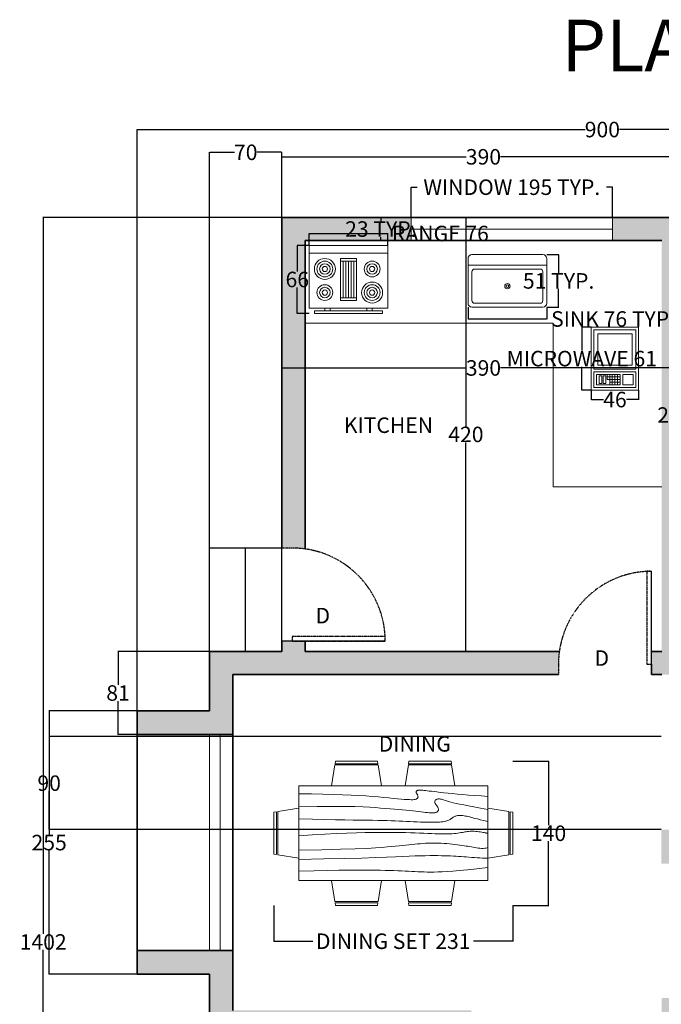
# Model space of a CAD drawing. Units: centimetres. Extents: x 355 to 1615, y 1030 to 2729.
# Tile 2 of 3: x 358 to 978, y 1776 to 2729. Entities that reach past the tile are written whole.
import ezdxf

# ---------------------------------------------------------------- set-up
doc = ezdxf.new("R2010")
doc.units = ezdxf.units.CM
doc.header["$MEASUREMENT"] = 0
doc.linetypes.add('HIDDEN', pattern=[0.375, 0.25, -0.125])
for name, color, linetype, lineweight in [('A-ANNO-DIMS', 2, 'Continuous', 18), ('A-ANNO-TEXT', 7, 'Continuous', 25), ('A-AREA-IDEN', 7, 'Continuous', 25), ('A-DOOR', 4, 'Continuous', 25), ('A-DOOR-HIDN', 4, 'HIDDEN', 25), ('A-EQPM', 8, 'Continuous', 18), ('A-FLOR-CASE', 9, 'Continuous', 20), ('A-FLOR-FIXT', 9, 'Continuous', 18), ('A-FLOR-STRS', 7, 'Continuous', 25), ('A-FURN', 8, 'Continuous', 18), ('A-GLAZ', 4, 'Continuous', 18), ('A-WALL', 7, 'Continuous', 35), ('A-WALL-PATT', 5, 'Continuous', 13)]:
    doc.layers.add(name, color=color, linetype=linetype, lineweight=lineweight)
doc.styles.get("Standard").update_dxf_attribs({"font": 'arial.ttf'})
doc.dimstyles.get("Standard").update_dxf_attribs({"dimtxt": 15, "dimasz": 0.18, "dimexe": 0.18, "dimexo": 0.0625, "dimgap": 0.09, "dimtad": 0, "dimtih": 1, "dimtoh": 1, "dimdec": 0, "dimzin": 0, "dimdsep": 46, "dimtxsty": 'Standard', "dimcen": 0.09, "dimadec": 0, "dimazin": 0, "dimtfac": 1, "dimtdec": 0, "dimtofl": 0, "dimtmove": 0, "dimatfit": 3, "dimfxl": 1, "dimtolj": 1, "dimtzin": 0, "dimarcsym": 0})

# ---------------------------------------------------------------- blocks, each defined once
blk = doc.blocks.new('*U2')
for p, q in [((0, 0), (0, -100)), ((-900, 0), (-900, -100))]:
    blk.add_line(p, q)
blk.add_lwpolyline([(0, 0), (0, 900), (-43.75, 900), (-43.75, 0)], close=True)
blk.add_arc((0, 0), 900, 90, 180)
blk = doc.blocks.new('*U3')
for p, q in [((0, 0), (0, -100)), ((-900, 0), (-900, -100))]:
    blk.add_line(p, q)
blk.add_lwpolyline([(0, 0), (0, 900), (-43.75, 900), (-43.75, 0)], close=True)
blk.add_arc((0, 0), 900, 90, 180)
blk = doc.blocks.new('Range-Oven - 30 in top')
for p, q in [((0, -3), (30, -3)), ((12, -6), (18, -6)), ((13, -20), (13, -6)), ((14, -6), (14, -20)), ((15, -20), (15, -6)), ((16, -6), (16, -20)), ((17, -20), (17, -6)), ((18, -20), (12, -20)), ((6, -24), (6, -25)), ((8, -25), (8, -24)), ((22, -25), (22, -24)), ((24, -24), (24, -25))]:
    blk.add_line(p, q)
for points in [[(0, -24), (0, 0), (30, 0), (30, -24)], [(12, -21), (12, -5), (18, -5), (18, -21)], [(2, -26), (2, -25), (28, -25), (28, -26)]]:
    blk.add_lwpolyline(points, close=True)
for centre, radius in [((6, -9), 4), ((6, -9), 3), ((6, -9), 2), ((24, -9), 3), ((24, -9), 2), ((6, -9), 1), ((24, -9), 1), ((6, -18), 3), ((24, -18), 4), ((24, -18), 3), ((6, -18), 2), ((6, -18), 1), ((24, -18), 2), ((24, -18), 1)]:
    blk.add_circle(centre, radius)
blk = doc.blocks.new('Sink-single - 30 in top')
blk.add_line((-15, -3.999996), (15, -3.999996))
for points in [[(-13.5, 0), (13.5, 0)], [(-15, -18.499996), (-15, -1.5)], [(15, -1.5), (15, -18.499996)], [(-13.5, -17.499996), (-13.5, -6.499996)], [(-12.5, -5.499996), (12.5, -5.499996)], [(13.5, -6.499996), (13.5, -17.499996)], [(12.5, -18.499996), (-12.5, -18.499996)], [(13.5, -19.999996), (-13.5, -19.999996)]]:
    blk.add_lwpolyline(points)
for radius in [1, 0.5]:
    blk.add_circle((0, -11.999996), radius)
for centre, radius, start, end in [((-13.5, -1.5), 1.5, 90, 180), ((13.5, -1.5), 1.5, 0, 90), ((-12.5, -6.499996), 1, 90, 180), ((12.5, -6.499996), 1, 0, 90), ((-13.5, -18.499996), 1.5, 180, 270), ((-12.5, -17.499996), 1, 180, 270), ((12.5, -17.499996), 1, 270, 0), ((13.5, -18.499996), 1.5, 270, 0)]:
    blk.add_arc(centre, radius, start, end)
blk = doc.blocks.new('Microwave')
for p, q in [((18, 10), (22, 10)), ((22, 9), (18, 9)), ((18, 8), (22, 8)), ((19, 7), (19, 11)), ((20, 11), (20, 7)), ((21, 7), (21, 11)), ((22, 7), (18, 7)), ((20, 6), (18, 6)), ((19, 6), (19, 7)), ((20, 7), (20, 6))]:
    blk.add_line(p, q)
for points in [[(0, 0), (0, 18), (24, 18), (24, 0)], [(1, 1), (1, 17), (16, 17), (16, 1)], [(2.5, 2.5), (2.5, 15.5), (14.5, 15.5), (14.5, 2.5)], [(17, 1), (17, 17), (23, 17), (23, 1)], [(18, 12), (18, 16), (22, 16), (22, 12)], [(18, 2), (18, 11), (22, 11), (22, 2)], [(18.5, 4.5), (18.5, 5.5), (21.5, 5.5), (21.5, 4.5)], [(18.5, 3), (18.5, 4), (21.5, 4), (21.5, 3)]]:
    blk.add_lwpolyline(points, close=True)
blk = doc.blocks.new('*D8')
at = {"layer": 'A-ANNO-DIMS', "color": 0, "lineweight": -2, "transparency": 16777216}
for p, q in [((611.23, 2537.61), (611.23, 2391.81)), ((1001.23, 2537.61), (1001.23, 2391.81)), ((611.41, 2391.99), (789.6, 2391.99)), ((1001.05, 2391.99), (822.86, 2391.99))]:
    blk.add_line(p, q, dxfattribs=at)
at = {"layer": 'A-ANNO-DIMS', "color": 0, "transparency": 16777216}
for points in [[(611.41, 2392.02), (611.41, 2391.96), (611.23, 2391.99)], [(1001.05, 2392.02), (1001.05, 2391.96), (1001.23, 2391.99)]]:
    blk.add_solid(points, dxfattribs=at)
at = {"layer": 'Defpoints', "color": 0, "transparency": 16777216}
for p in [(611.23, 2537.67), (1001.23, 2537.67), (1001.23, 2391.99)]:
    blk.add_point(p, dxfattribs=at)
at = {"layer": 'A-ANNO-DIMS', "color": 0, "transparency": 16777216, "insert": (806.23, 2391.99), "char_height": 15, "attachment_point": 5}
blk.add_mtext('\\A1;390', dxfattribs=at)
blk = doc.blocks.new('*D9')
at = {"layer": 'A-ANNO-DIMS', "color": 0, "lineweight": -2, "transparency": 16777216}
for p, q in [((765.93, 2537.67), (789.45, 2537.67)), ((789.27, 2537.49), (789.27, 2335.42)), ((789.27, 2117.85), (789.27, 2319.92)), ((765.93, 2117.67), (789.45, 2117.67))]:
    blk.add_line(p, q, dxfattribs=at)
at = {"layer": 'A-ANNO-DIMS', "color": 0, "transparency": 16777216}
for points in [[(789.24, 2537.49), (789.3, 2537.49), (789.27, 2537.67)], [(789.24, 2117.85), (789.3, 2117.85), (789.27, 2117.67)]]:
    blk.add_solid(points, dxfattribs=at)
at = {"layer": 'Defpoints', "color": 0, "transparency": 16777216}
for p in [(765.87, 2537.67), (765.87, 2117.67), (789.27, 2117.67)]:
    blk.add_point(p, dxfattribs=at)
at = {"layer": 'A-ANNO-DIMS', "color": 0, "transparency": 16777216, "insert": (789.27, 2327.67), "char_height": 15, "attachment_point": 5}
blk.add_mtext('\\A1;420', dxfattribs=at)
blk = doc.blocks.new('Dining Set - 36 x 72 in.')
for p, q in [((-22, 27.5), (-22.1562, 26.50042)), ((-5.8416, 26.5), (-22.1534, 26.5)), ((-22, 27.5), (-6, 27.5)), ((-5.8437, 26.49966), (-6, 27.5)), ((6, 27.5), (5.8438, 26.50042)), ((22.1584, 26.5), (5.8466, 26.5)), ((6, 27.5), (22, 27.5)), ((22.1563, 26.49966), (22, 27.5)), ((-22.2343, 26.00059), (-23.4847, 17.99762)), ((-22.2304, 26), (-5.7608, 26)), ((-4.5152, 17.99762), (-5.7655, 25.99926)), ((5.7657, 26.00059), (4.5153, 17.99762)), ((5.7696, 26), (22.2392, 26)), ((23.4848, 17.99762), (22.2345, 25.99926)), ((36, 18), (-36, 18)), ((-36, 18), (-36, -18)), ((36, -18), (36, 18)), ((-45.5, 8), (-44.5004, 8.15617)), ((-45.5, 8), (-45.5, -8)), ((-44.5, -8.15843), (-44.5, 8.15338)), ((-44.0006, 8.23428), (-35.9976, 9.48474)), ((-44, 8.23041), (-44, -8.23915)), ((44.0006, 8.23428), (35.9976, 9.48474)), ((44, 8.23041), (44, -8.23915)), ((44.5, -8.15843), (44.5, 8.15338)), ((45.5, 8), (44.5005, 8.15617)), ((45.5, 8), (45.5, -8)), ((-44.4997, -8.15631), (-45.5, -8)), ((-35.9976, -9.48476), (-43.9993, -8.2345)), ((35.9976, -9.48476), (43.9993, -8.2345)), ((44.4997, -8.15631), (45.5, -8)), ((-36, -18), (36, -18)), ((-22.2343, -26.0006), (-23.4847, -17.99762)), ((-4.5152, -17.99762), (-5.7655, -25.99928)), ((5.7657, -26.0006), (4.5153, -17.99762)), ((23.4848, -17.99762), (22.2345, -25.99928)), ((-22.2304, -26), (-5.7608, -26)), ((5.7696, -26), (22.2392, -26)), ((-22, -27.5), (-22.1562, -26.50044)), ((-5.8416, -26.5), (-22.1534, -26.5)), ((-22, -27.5), (-6, -27.5)), ((-5.8437, -26.49967), (-6, -27.5)), ((6, -27.5), (5.8438, -26.50044)), ((22.1584, -26.5), (5.8466, -26.5)), ((6, -27.5), (22, -27.5)), ((22.1563, -26.49967), (22, -27.5))]:
    blk.add_line(p, q)
for points in [[(-36, 15), (-31.1772, 14.97754), (-26.8079, 14.91406), (-22.8538, 14.81543), (-19.276, 14.6875), (-16.0362, 14.53613), (-13.0957, 14.36718), (-10.4159, 14.18652), (-7.9583, 14), (-5.6904, 13.81315), (-3.6035, 13.63021), (-1.6954, 13.45508), (0.0365, 13.29166), (1.5945, 13.14388), (2.9811, 13.01562), (4.1988, 12.9108), (5.25, 12.83333), (6.1393, 12.78613), (6.8802, 12.76823), (7.4883, 12.77767), (7.9792, 12.8125), (8.3685, 12.87077), (8.6719, 12.95052), (8.9049, 13.0498), (9.0833, 13.16666), (9.2205, 13.29899), (9.3216, 13.44401), (9.3895, 13.59879), (9.4271, 13.76041), (9.4373, 13.92594), (9.4232, 14.09245), (9.3875, 14.257), (9.3333, 14.41666), (9.2638, 14.56917), (9.1836, 14.71484), (9.0975, 14.85465), (9.0104, 14.98958), (8.9272, 15.1206), (8.8529, 15.2487), (8.7922, 15.37483), (8.75, 15.5), (8.7305, 15.62467), (8.7344, 15.74739), (8.7617, 15.86621), (8.8125, 15.97916), (8.8867, 16.08431), (8.9844, 16.17968), (9.1055, 16.26334), (9.25, 16.33333), (9.4189, 16.38802), (9.6172, 16.42708), (9.8506, 16.45052), (10.125, 16.45833), (10.4463, 16.45052), (10.8203, 16.42708), (11.2529, 16.38802), (11.75, 16.33333), (12.3184, 16.26318), (12.9694, 16.17838), (13.7151, 16.07991), (14.5677, 15.96875), (15.5395, 15.84586), (16.6426, 15.71224), (17.8893, 15.56884), (19.2917, 15.41666), (20.859, 15.25667), (22.5879, 15.08984), (24.4721, 14.91715), (26.5052, 14.73958), (28.6809, 14.5581), (30.9929, 14.3737), (33.4347, 14.18733), (36, 14)], [(-36, 10), (-28.9766, 10.14274), (-23.1725, 10.20442), (-18.4241, 10.19775), (-14.5677, 10.13541), (-11.4399, 10.03011), (-8.877, 9.89453), (-6.7154, 9.74137), (-4.7917, 9.58333), (-2.9698, 9.43082), (-1.2246, 9.28515), (0.4415, 9.14534), (2.026, 9.01041), (3.5266, 8.87939), (4.9408, 8.7513), (6.266, 8.62516), (7.5, 8.5), (8.6411, 8.37549), (9.6914, 8.2539), (10.6538, 8.13818), (11.5312, 8.03125), (12.3267, 7.93603), (13.043, 7.85547), (13.6831, 7.79248), (14.25, 7.75), (14.7471, 7.7303), (15.1797, 7.73307), (15.5537, 7.75732), (15.875, 7.80208), (16.1494, 7.86637), (16.3828, 7.94922), (16.5811, 8.04964), (16.75, 8.16666), (16.8944, 8.29915), (17.0143, 8.44531), (17.1089, 8.60319), (17.1771, 8.77083), (17.218, 8.94629), (17.2305, 9.1276), (17.2137, 9.31282), (17.1667, 9.5), (17.0895, 9.6875), (16.987, 9.875), (16.8649, 10.0625), (16.7292, 10.25), (16.5856, 10.4375), (16.4401, 10.625), (16.2985, 10.8125), (16.1667, 11), (16.05, 11.18733), (15.9518, 11.3737), (15.8752, 11.5581), (15.8229, 11.73958), (15.798, 11.91715), (15.8034, 12.08984), (15.842, 12.25667), (15.9167, 12.41666), (16.0295, 12.56836), (16.1784, 12.70833), (16.3605, 12.83268), (16.5729, 12.9375), (16.8127, 13.01888), (17.0768, 13.07291), (17.3625, 13.0957), (17.6667, 13.08333), (17.9894, 13.03312), (18.3418, 12.94726), (18.7382, 12.82918), (19.1927, 12.68229), (19.7195, 12.51001), (20.3327, 12.31575), (21.0465, 12.10294), (21.875, 11.875), (22.8357, 11.63354), (23.959, 11.37304), (25.2786, 11.08618), (26.8282, 10.76562), (28.6414, 10.40405), (30.752, 9.99414), (33.1936, 9.52856), (36, 9)], [(-36, 5.5), (-30.7157, 5.3348), (-26.069, 5.20963), (-21.9946, 5.11767), (-18.4271, 5.05208), (-15.3009, 5.00602), (-12.5508, 4.97265), (-10.1112, 4.94515), (-7.9167, 4.91666), (-5.909, 4.88167), (-4.0586, 4.83984), (-2.3429, 4.79215), (-0.7396, 4.73958), (0.7739, 4.6831), (2.22, 4.6237), (3.6213, 4.56233), (5, 4.5), (6.373, 4.43782), (7.7344, 4.3776), (9.0723, 4.32129), (10.375, 4.27083), (11.6309, 4.22819), (12.8281, 4.19531), (13.9551, 4.17415), (15, 4.16666), (15.954, 4.17448), (16.819, 4.19791), (17.6001, 4.23698), (18.3021, 4.29166), (18.9299, 4.36198), (19.4883, 4.44791), (19.9823, 4.54948), (20.4167, 4.66666), (20.7969, 4.79899), (21.1302, 4.94401), (21.4245, 5.09879), (21.6875, 5.26041), (21.9271, 5.42594), (22.1511, 5.59245), (22.3672, 5.757), (22.5834, 5.91666), (22.8065, 6.06868), (23.0404, 6.21093), (23.2879, 6.34147), (23.5521, 6.45833), (23.8358, 6.55957), (24.142, 6.64323), (24.4735, 6.70735), (24.8334, 6.75), (25.2235, 6.76969), (25.642, 6.76692), (26.0858, 6.74267), (26.5521, 6.69791), (27.0379, 6.63362), (27.5404, 6.55078), (28.0565, 6.45036), (28.5834, 6.33333), (29.1242, 6.19987), (29.7071, 6.04687), (30.3661, 5.87044), (31.1354, 5.66666), (32.0493, 5.43164), (33.142, 5.16146), (34.4475, 4.85221), (36, 4.5)], [(-36, -1), (-30.7915, -0.6591), (-26.0195, -0.38216), (-21.6519, -0.16284), (-17.6563, 0.00521), (-14.0005, 0.12833), (-10.6523, 0.21289), (-7.5796, 0.26522), (-4.75, 0.29166), (-2.134, 0.29793), (0.2878, 0.28711), (2.5317, 0.26163), (4.6146, 0.22396), (6.5529, 0.17651), (8.3633, 0.12174), (10.0623, 0.06209), (11.6667, 0), (13.1899, -0.06201), (14.6341, -0.1211), (15.9982, -0.17432), (17.2813, -0.21875), (18.4823, -0.25147), (19.6003, -0.26953), (20.6343, -0.27002), (21.5834, -0.25), (22.4481, -0.20768), (23.2357, -0.14584), (23.9549, -0.06836), (24.6146, 0.02083), (25.2235, 0.11784), (25.7904, 0.21875), (26.3241, 0.31966), (26.8334, 0.41666), (27.3265, 0.50618), (27.8099, 0.58593), (28.2894, 0.65397), (28.7709, 0.70833), (29.2601, 0.74707), (29.763, 0.76823), (30.2855, 0.76985), (30.8334, 0.75), (31.4088, 0.70784), (31.9994, 0.64713), (32.589, 0.57275), (33.1615, 0.48958), (33.7008, 0.4025), (34.1908, 0.3164), (34.6153, 0.23616), (34.9584, 0.16666), (35.2099, 0.11165), (35.3848, 0.07031), (35.504, 0.04069), (35.5886, 0.02083), (35.6594, 0.00879), (35.7377, 0.0026), (35.8442, 0.00032), (36, 0)], [(-36, -6.5), (-27.1843, -6.31267), (-20.084, -6.1263), (-14.469, -5.9419), (-10.1094, -5.76042), (-6.7752, -5.58285), (-4.2363, -5.41016), (-2.2629, -5.24333), (-0.625, -5.08334), (0.8708, -4.93099), (2.2715, -4.78646), (3.5872, -4.64974), (4.8281, -4.52084), (6.0046, -4.39974), (7.127, -4.28646), (8.2053, -4.18099), (9.25, -4.08334), (10.2705, -3.99382), (11.2734, -3.91407), (12.2647, -3.84603), (13.25, -3.79167), (14.2354, -3.75293), (15.2266, -3.73177), (16.2295, -3.73015), (17.25, -3.75), (18.2912, -3.79248), (19.3451, -3.85547), (20.4009, -3.93604), (21.4479, -4.03125), (22.4754, -4.13819), (23.4727, -4.25391), (24.4289, -4.37549), (25.3334, -4.5), (26.1785, -4.62492), (26.9694, -4.74935), (27.7145, -4.87281), (28.4219, -4.99479), (29.1, -5.11483), (29.7572, -5.23242), (30.4016, -5.34709), (31.0417, -5.45834), (31.6837, -5.56437), (32.3262, -5.65821), (32.9658, -5.73153), (33.599, -5.77604), (34.2224, -5.78345), (34.8327, -5.74545), (35.4264, -5.65373), (36, -5.5)], [(-36, -10), (-26.4022, -9.81299), (-18.4675, -9.62891), (-11.9839, -9.45069), (-6.7396, -9.28125), (-2.5226, -9.12354), (0.8789, -8.98047), (3.6769, -8.85498), (6.0833, -8.75), (8.2767, -8.66765), (10.3021, -8.60677), (12.1712, -8.56543), (13.8958, -8.54167), (15.4876, -8.53353), (16.9583, -8.53907), (18.3197, -8.55632), (19.5834, -8.58334), (20.7616, -8.61841), (21.8685, -8.66081), (22.9188, -8.71004), (23.9271, -8.76563), (24.9081, -8.82707), (25.8763, -8.89388), (26.8465, -8.96558), (27.8334, -9.04167), (28.8474, -9.12118), (29.8828, -9.20117), (30.93, -9.27824), (31.9792, -9.34896), (33.0205, -9.40991), (34.0443, -9.45768), (35.0407, -9.48885), (36, -9.5)], [(-36, -14.5), (-30.0881, -14.33513), (-25.0332, -14.21224), (-20.7312, -14.12647), (-17.0781, -14.07292), (-13.97, -14.04671), (-11.3027, -14.04297), (-8.9724, -14.05681), (-6.875, -14.08334), (-4.9224, -14.11833), (-3.0905, -14.16016), (-1.3709, -14.20785), (0.2448, -14.26042), (1.7647, -14.3169), (3.1973, -14.3763), (4.5507, -14.43767), (5.8333, -14.5), (7.0554, -14.5621), (8.235, -14.62175), (9.3922, -14.67652), (10.5469, -14.72396), (11.7192, -14.76164), (12.929, -14.78711), (14.1965, -14.79794), (15.5417, -14.79167), (16.9933, -14.76424), (18.6152, -14.70508), (20.4804, -14.60197), (22.6615, -14.44271), (25.2312, -14.21509), (28.2624, -13.9069), (31.8277, -13.50594), (36, -13)]]:
    blk.add_lwpolyline(points)
blk = doc.blocks.new('*D23')
at = {"layer": 'A-ANNO-DIMS', "color": 0, "lineweight": -2, "transparency": 16777216}
for p, q in [((541.41, 2217.73), (541.41, 2600.88)), ((541.59, 2600.7), (565.58, 2600.7)), ((611.05, 2600.7), (587.07, 2600.7)), ((611.23, 2217.73), (611.23, 2600.88))]:
    blk.add_line(p, q, dxfattribs=at)
at = {"layer": 'A-ANNO-DIMS', "color": 0, "transparency": 16777216}
for points in [[(541.59, 2600.73), (541.59, 2600.67), (541.41, 2600.7)], [(611.05, 2600.73), (611.05, 2600.67), (611.23, 2600.7)]]:
    blk.add_solid(points, dxfattribs=at)
at = {"layer": 'Defpoints', "color": 0, "transparency": 16777216}
for p in [(611.23, 2600.7), (541.41, 2217.67), (611.23, 2217.67)]:
    blk.add_point(p, dxfattribs=at)
at = {"layer": 'A-ANNO-DIMS', "color": 0, "transparency": 16777216, "insert": (576.32, 2600.7), "char_height": 15, "attachment_point": 5}
blk.add_mtext('\\A1;70', dxfattribs=at)
blk = doc.blocks.new('*D24')
at = {"layer": 'A-ANNO-DIMS', "color": 0, "lineweight": -2, "transparency": 16777216}
for p, q in [((611.23, 2537.73), (611.23, 2596.51)), ((611.41, 2596.33), (789.6, 2596.33)), ((1001.05, 2596.33), (822.86, 2596.33)), ((1001.23, 2537.73), (1001.23, 2596.51))]:
    blk.add_line(p, q, dxfattribs=at)
at = {"layer": 'A-ANNO-DIMS', "color": 0, "transparency": 16777216}
for points in [[(611.41, 2596.36), (611.41, 2596.3), (611.23, 2596.33)], [(1001.05, 2596.36), (1001.05, 2596.3), (1001.23, 2596.33)]]:
    blk.add_solid(points, dxfattribs=at)
at = {"layer": 'Defpoints', "color": 0, "transparency": 16777216}
for p in [(1001.23, 2596.33), (611.23, 2537.67), (1001.23, 2537.67)]:
    blk.add_point(p, dxfattribs=at)
at = {"layer": 'A-ANNO-DIMS', "color": 0, "transparency": 16777216, "insert": (806.23, 2596.33), "char_height": 15, "attachment_point": 5}
blk.add_mtext('\\A1;390', dxfattribs=at)
blk = doc.blocks.new('*D31')
at = {"layer": 'A-ANNO-DIMS', "color": 0, "lineweight": -2, "transparency": 16777216}
for p, q in [((611.17, 2537.67), (380.23, 2537.67)), ((380.41, 2537.49), (380.41, 1844.25)), ((380.41, 1135.51), (380.41, 1828.75)), ((541.17, 1135.33), (380.23, 1135.33))]:
    blk.add_line(p, q, dxfattribs=at)
at = {"layer": 'A-ANNO-DIMS', "color": 0, "transparency": 16777216}
for points in [[(380.38, 2537.49), (380.44, 2537.49), (380.41, 2537.67)], [(380.38, 1135.51), (380.44, 1135.51), (380.41, 1135.33)]]:
    blk.add_solid(points, dxfattribs=at)
at = {"layer": 'Defpoints', "color": 0, "transparency": 16777216}
for p in [(380.41, 2537.67), (611.23, 2537.67), (541.23, 1135.33)]:
    blk.add_point(p, dxfattribs=at)
at = {"layer": 'A-ANNO-DIMS', "color": 0, "transparency": 16777216, "insert": (380.41, 1836.5), "char_height": 15, "attachment_point": 5}
blk.add_mtext('\\A1;1402', dxfattribs=at)
blk = doc.blocks.new('*D32')
at = {"layer": 'A-ANNO-DIMS', "color": 0, "lineweight": -2, "transparency": 16777216}
for p, q in [((541.17, 2117.67), (452.64, 2117.67)), ((452.82, 2117.49), (452.82, 2085.17)), ((452.82, 2037.35), (452.82, 2069.67)), ((541.17, 2037.17), (452.64, 2037.17))]:
    blk.add_line(p, q, dxfattribs=at)
at = {"layer": 'A-ANNO-DIMS', "color": 0, "transparency": 16777216}
for points in [[(452.79, 2117.49), (452.85, 2117.49), (452.82, 2117.67)], [(452.79, 2037.35), (452.85, 2037.35), (452.82, 2037.17)]]:
    blk.add_solid(points, dxfattribs=at)
at = {"layer": 'Defpoints', "color": 0, "transparency": 16777216}
for p in [(541.23, 2117.67), (452.82, 2037.17), (541.23, 2037.17)]:
    blk.add_point(p, dxfattribs=at)
at = {"layer": 'A-ANNO-DIMS', "color": 0, "transparency": 16777216, "insert": (452.82, 2077.42), "char_height": 15, "attachment_point": 5}
blk.add_mtext('\\A1;81', dxfattribs=at)
blk = doc.blocks.new('WIN-1949')
blk.add_line((194.84, 11.25), (0, 11.25))
blk.add_lwpolyline([(0, 22.5), (194.84, 22.5), (194.84, 0), (0, 0)], close=True)
blk = doc.blocks.new('*D39')
at = {"layer": 'A-ANNO-DIMS', "color": 0, "lineweight": -2, "transparency": 16777216}
for p, q in [((1024.6, 2357.67), (1008.67, 2357.67)), ((1008.85, 2357.49), (1008.85, 2354.17)), ((1024.6, 2335.17), (1008.67, 2335.17)), ((1008.85, 2335.35), (1008.85, 2338.67))]:
    blk.add_line(p, q, dxfattribs=at)
at = {"layer": 'A-ANNO-DIMS', "color": 0, "transparency": 16777216}
for points in [[(1008.82, 2357.49), (1008.88, 2357.49), (1008.85, 2357.67)], [(1008.82, 2335.35), (1008.88, 2335.35), (1008.85, 2335.17)]]:
    blk.add_solid(points, dxfattribs=at)
at = {"layer": 'Defpoints', "color": 0, "transparency": 16777216}
for p in [(1008.85, 2357.67), (1024.66, 2357.67), (1024.66, 2335.17)]:
    blk.add_point(p, dxfattribs=at)
at = {"layer": 'A-ANNO-DIMS', "color": 0, "transparency": 16777216, "insert": (1008.85, 2346.42), "char_height": 15, "attachment_point": 5}
blk.add_mtext('\\A1;23 TYP.', dxfattribs=at)
blk = doc.blocks.new('*D42')
at = {"layer": 'A-ANNO-DIMS', "color": 0, "lineweight": -2, "transparency": 16777216}
for p, q in [((736.23, 2537.73), (736.23, 2567.08)), ((736.41, 2566.9), (742.04, 2566.9)), ((930.89, 2566.9), (925.27, 2566.9)), ((931.07, 2537.73), (931.07, 2567.08))]:
    blk.add_line(p, q, dxfattribs=at)
at = {"layer": 'A-ANNO-DIMS', "color": 0, "transparency": 16777216}
for points in [[(736.41, 2566.93), (736.41, 2566.87), (736.23, 2566.9)], [(930.89, 2566.93), (930.89, 2566.87), (931.07, 2566.9)]]:
    blk.add_solid(points, dxfattribs=at)
at = {"layer": 'Defpoints', "color": 0, "transparency": 16777216}
for p in [(931.07, 2566.9), (736.23, 2537.67), (931.07, 2537.67)]:
    blk.add_point(p, dxfattribs=at)
at = {"layer": 'A-ANNO-DIMS', "color": 0, "transparency": 16777216, "insert": (833.65, 2566.9), "char_height": 15, "attachment_point": 5}
blk.add_mtext('\\A1;WINDOW 195 TYP.', dxfattribs=at)
blk = doc.blocks.new('*D43')
at = {"layer": 'A-ANNO-DIMS', "color": 0, "lineweight": -2, "transparency": 16777216}
for p, q in [((736.17, 2537.67), (706.83, 2537.67)), ((707.01, 2537.49), (707.01, 2534.17)), ((707.01, 2515.35), (707.01, 2518.67)), ((736.17, 2515.17), (706.83, 2515.17))]:
    blk.add_line(p, q, dxfattribs=at)
at = {"layer": 'A-ANNO-DIMS', "color": 0, "transparency": 16777216}
for points in [[(706.98, 2537.49), (707.04, 2537.49), (707.01, 2537.67)], [(706.98, 2515.35), (707.04, 2515.35), (707.01, 2515.17)]]:
    blk.add_solid(points, dxfattribs=at)
at = {"layer": 'Defpoints', "color": 0, "transparency": 16777216}
for p in [(707.01, 2537.67), (736.23, 2537.67), (736.23, 2515.17)]:
    blk.add_point(p, dxfattribs=at)
at = {"layer": 'A-ANNO-DIMS', "color": 0, "transparency": 16777216, "insert": (707.01, 2526.42), "char_height": 15, "attachment_point": 5}
blk.add_mtext('\\A1;23 TYP.', dxfattribs=at)
blk = doc.blocks.new('*D44')
at = {"layer": 'A-ANNO-DIMS', "color": 0, "lineweight": -2, "transparency": 16777216}
for p, q in [((791.29, 2450.77), (791.29, 2439.22)), ((867.49, 2450.77), (867.49, 2439.22)), ((791.47, 2439.4), (867.31, 2439.4)), ((867.49, 2439.4), (867.67, 2439.4))]:
    blk.add_line(p, q, dxfattribs=at)
at = {"layer": 'A-ANNO-DIMS', "color": 0, "transparency": 16777216}
for points in [[(791.47, 2439.43), (791.47, 2439.37), (791.29, 2439.4)], [(867.31, 2439.43), (867.31, 2439.37), (867.49, 2439.4)]]:
    blk.add_solid(points, dxfattribs=at)
at = {"layer": 'Defpoints', "color": 0, "transparency": 16777216}
for p in [(791.29, 2450.83), (867.49, 2450.83), (867.49, 2439.4)]:
    blk.add_point(p, dxfattribs=at)
at = {"layer": 'A-ANNO-DIMS', "color": 0, "transparency": 16777216, "insert": (931.59, 2439.4), "char_height": 15, "attachment_point": 5}
blk.add_mtext('\\A1;SINK 76 TYP.', dxfattribs=at)
blk = doc.blocks.new('*D45')
at = {"layer": 'A-ANNO-DIMS', "color": 0, "lineweight": -2, "transparency": 16777216}
for p, q in [((867.55, 2501.63), (879.1, 2501.63)), ((878.92, 2501.45), (878.92, 2483.98)), ((878.92, 2451.01), (878.92, 2468.48)), ((867.55, 2450.83), (879.1, 2450.83))]:
    blk.add_line(p, q, dxfattribs=at)
at = {"layer": 'A-ANNO-DIMS', "color": 0, "transparency": 16777216}
for points in [[(878.89, 2501.45), (878.95, 2501.45), (878.92, 2501.63)], [(878.89, 2451.01), (878.95, 2451.01), (878.92, 2450.83)]]:
    blk.add_solid(points, dxfattribs=at)
at = {"layer": 'Defpoints', "color": 0, "transparency": 16777216}
for p in [(867.49, 2501.63), (878.92, 2501.63), (867.49, 2450.83)]:
    blk.add_point(p, dxfattribs=at)
at = {"layer": 'A-ANNO-DIMS', "color": 0, "transparency": 16777216, "insert": (878.92, 2476.23), "char_height": 15, "attachment_point": 5}
blk.add_mtext('\\A1;51 TYP.', dxfattribs=at)
blk = doc.blocks.new('*D50')
at = {"layer": 'A-ANNO-DIMS', "color": 0, "lineweight": -2, "transparency": 16777216}
for p, q in [((637.6, 2510.71), (637.6, 2522.26)), ((637.78, 2522.08), (713.62, 2522.08)), ((713.8, 2510.71), (713.8, 2522.26)), ((713.8, 2522.08), (713.98, 2522.08))]:
    blk.add_line(p, q, dxfattribs=at)
at = {"layer": 'A-ANNO-DIMS', "color": 0, "transparency": 16777216}
for points in [[(637.78, 2522.11), (637.78, 2522.05), (637.6, 2522.08)], [(713.62, 2522.11), (713.62, 2522.05), (713.8, 2522.08)]]:
    blk.add_solid(points, dxfattribs=at)
at = {"layer": 'Defpoints', "color": 0, "transparency": 16777216}
for p in [(713.8, 2522.08), (637.6, 2510.65), (713.8, 2510.65)]:
    blk.add_point(p, dxfattribs=at)
at = {"layer": 'A-ANNO-DIMS', "color": 0, "transparency": 16777216, "insert": (764.59, 2522.08), "char_height": 15, "attachment_point": 5}
blk.add_mtext('\\A1;RANGE 76', dxfattribs=at)
blk = doc.blocks.new('*D51')
at = {"layer": 'A-ANNO-DIMS', "color": 0, "lineweight": -2, "transparency": 16777216}
for p, q in [((637.54, 2510.65), (625.99, 2510.65)), ((626.17, 2510.47), (626.17, 2485.38)), ((626.17, 2444.79), (626.17, 2469.88)), ((637.54, 2444.61), (625.99, 2444.61))]:
    blk.add_line(p, q, dxfattribs=at)
at = {"layer": 'A-ANNO-DIMS', "color": 0, "transparency": 16777216}
for points in [[(626.14, 2510.47), (626.2, 2510.47), (626.17, 2510.65)], [(626.14, 2444.79), (626.2, 2444.79), (626.17, 2444.61)]]:
    blk.add_solid(points, dxfattribs=at)
at = {"layer": 'Defpoints', "color": 0, "transparency": 16777216}
for p in [(626.17, 2510.65), (637.6, 2510.65), (637.6, 2444.61)]:
    blk.add_point(p, dxfattribs=at)
at = {"layer": 'A-ANNO-DIMS', "color": 0, "transparency": 16777216, "insert": (626.17, 2477.63), "char_height": 15, "attachment_point": 5}
blk.add_mtext('\\A1;66', dxfattribs=at)
blk = doc.blocks.new('*D52')
at = {"layer": 'A-ANNO-DIMS', "color": 0, "lineweight": -2, "transparency": 16777216}
for p, q in [((910.47, 2431.5), (901.2, 2431.5)), ((901.38, 2431.32), (901.38, 2408.87)), ((901.38, 2370.72), (901.38, 2393.17)), ((910.47, 2370.54), (901.2, 2370.54))]:
    blk.add_line(p, q, dxfattribs=at)
at = {"layer": 'A-ANNO-DIMS', "color": 0, "transparency": 16777216}
for points in [[(901.35, 2431.32), (901.41, 2431.32), (901.38, 2431.5)], [(901.35, 2370.72), (901.41, 2370.72), (901.38, 2370.54)]]:
    blk.add_solid(points, dxfattribs=at)
at = {"layer": 'Defpoints', "color": 0, "transparency": 16777216}
for p in [(910.53, 2431.5), (901.38, 2370.54), (910.53, 2370.54)]:
    blk.add_point(p, dxfattribs=at)
at = {"layer": 'A-ANNO-DIMS', "color": 0, "transparency": 16777216, "insert": (901.38, 2401.02), "char_height": 15, "attachment_point": 5}
blk.add_mtext('\\A1;MICROWAVE 61', dxfattribs=at)
blk = doc.blocks.new('*D53')
at = {"layer": 'A-ANNO-DIMS', "color": 0, "lineweight": -2, "transparency": 16777216}
for p, q in [((910.53, 2370.47), (910.53, 2361.21)), ((956.25, 2370.47), (956.25, 2361.21)), ((910.71, 2361.39), (922.26, 2361.39)), ((956.07, 2361.39), (944.52, 2361.39))]:
    blk.add_line(p, q, dxfattribs=at)
at = {"layer": 'A-ANNO-DIMS', "color": 0, "transparency": 16777216}
for points in [[(910.71, 2361.42), (910.71, 2361.36), (910.53, 2361.39)], [(956.07, 2361.42), (956.07, 2361.36), (956.25, 2361.39)]]:
    blk.add_solid(points, dxfattribs=at)
at = {"layer": 'Defpoints', "color": 0, "transparency": 16777216}
for p in [(910.53, 2370.54), (956.25, 2370.54), (956.25, 2361.39)]:
    blk.add_point(p, dxfattribs=at)
at = {"layer": 'A-ANNO-DIMS', "color": 0, "transparency": 16777216, "insert": (933.39, 2361.39), "char_height": 15, "attachment_point": 5}
blk.add_mtext('\\A1;46', dxfattribs=at)
blk = doc.blocks.new('*D58')
at = {"layer": 'A-ANNO-DIMS', "color": 0, "lineweight": -2, "transparency": 16777216}
for p, q in [((603.4, 1871.81), (603.4, 1837.02)), ((834.54, 1871.81), (834.54, 1837.02)), ((603.58, 1837.2), (641.26, 1837.2)), ((834.36, 1837.2), (796.67, 1837.2))]:
    blk.add_line(p, q, dxfattribs=at)
at = {"layer": 'A-ANNO-DIMS', "color": 0, "transparency": 16777216}
for points in [[(603.58, 1837.23), (603.58, 1837.17), (603.4, 1837.2)], [(834.36, 1837.23), (834.36, 1837.17), (834.54, 1837.2)]]:
    blk.add_solid(points, dxfattribs=at)
at = {"layer": 'Defpoints', "color": 0, "transparency": 16777216}
for p in [(603.4, 1871.87), (834.54, 1871.87), (834.54, 1837.2)]:
    blk.add_point(p, dxfattribs=at)
at = {"layer": 'A-ANNO-DIMS', "color": 0, "transparency": 16777216, "insert": (718.97, 1837.2), "char_height": 15, "attachment_point": 5}
blk.add_mtext('\\A1;DINING SET 231', dxfattribs=at)
blk = doc.blocks.new('*D59')
at = {"layer": 'A-ANNO-DIMS', "color": 0, "lineweight": -2, "transparency": 16777216}
for p, q in [((834.6, 2011.57), (869.39, 2011.57)), ((869.21, 2011.39), (869.21, 1949.47)), ((869.21, 1872.05), (869.21, 1933.98)), ((834.6, 1871.87), (869.39, 1871.87))]:
    blk.add_line(p, q, dxfattribs=at)
at = {"layer": 'A-ANNO-DIMS', "color": 0, "transparency": 16777216}
for points in [[(869.18, 2011.39), (869.24, 2011.39), (869.21, 2011.57)], [(869.18, 1872.05), (869.24, 1872.05), (869.21, 1871.87)]]:
    blk.add_solid(points, dxfattribs=at)
at = {"layer": 'Defpoints', "color": 0, "transparency": 16777216}
for p in [(834.54, 2011.57), (869.21, 2011.57), (834.54, 1871.87)]:
    blk.add_point(p, dxfattribs=at)
at = {"layer": 'A-ANNO-DIMS', "color": 0, "transparency": 16777216, "insert": (869.21, 1941.72), "char_height": 15, "attachment_point": 5}
blk.add_mtext('\\A1;140', dxfattribs=at)
blk = doc.blocks.new('*D64')
at = {"layer": 'A-ANNO-DIMS', "color": 0, "lineweight": -2, "transparency": 16777216}
for p, q in [((471.23, 2060.23), (471.23, 2622.9)), ((471.41, 2622.72), (904.6, 2622.72)), ((1371.05, 2622.72), (937.87, 2622.72)), ((1371.23, 2357.73), (1371.23, 2622.9))]:
    blk.add_line(p, q, dxfattribs=at)
at = {"layer": 'A-ANNO-DIMS', "color": 0, "transparency": 16777216}
for points in [[(471.41, 2622.75), (471.41, 2622.69), (471.23, 2622.72)], [(1371.05, 2622.75), (1371.05, 2622.69), (1371.23, 2622.72)]]:
    blk.add_solid(points, dxfattribs=at)
at = {"layer": 'Defpoints', "color": 0, "transparency": 16777216}
for p in [(1371.23, 2622.72), (1371.23, 2357.67), (471.23, 2060.17)]:
    blk.add_point(p, dxfattribs=at)
at = {"layer": 'A-ANNO-DIMS', "color": 0, "transparency": 16777216, "insert": (921.23, 2622.72), "char_height": 15, "attachment_point": 5}
blk.add_mtext('\\A1;900', dxfattribs=at)
blk = doc.blocks.new('*D70')
at = {"layer": 'A-ANNO-DIMS', "color": 0, "lineweight": -2, "transparency": 16777216}
for p, q in [((978.17, 2035.17), (386, 2035.17)), ((386.18, 2034.99), (386.18, 1997.92)), ((386.18, 1945.35), (386.18, 1982.42)), ((978.17, 1945.17), (386, 1945.17))]:
    blk.add_line(p, q, dxfattribs=at)
at = {"layer": 'A-ANNO-DIMS', "color": 0, "transparency": 16777216}
for points in [[(386.15, 2034.99), (386.21, 2034.99), (386.18, 2035.17)], [(386.15, 1945.35), (386.21, 1945.35), (386.18, 1945.17)]]:
    blk.add_solid(points, dxfattribs=at)
at = {"layer": 'Defpoints', "color": 0, "transparency": 16777216}
for p in [(386.18, 2035.17), (978.23, 2035.17), (978.23, 1945.17)]:
    blk.add_point(p, dxfattribs=at)
at = {"layer": 'A-ANNO-DIMS', "color": 0, "transparency": 16777216, "insert": (386.18, 1990.17), "char_height": 15, "attachment_point": 5}
blk.add_mtext('\\A1;90', dxfattribs=at)
blk = doc.blocks.new('*D75')
at = {"layer": 'A-ANNO-DIMS', "color": 0, "lineweight": -2, "transparency": 16777216}
for p, q in [((471.17, 2060.17), (386, 2060.17)), ((386.18, 2059.99), (386.18, 1940.42)), ((386.18, 1805.35), (386.18, 1924.92)), ((471.17, 1805.17), (386, 1805.17))]:
    blk.add_line(p, q, dxfattribs=at)
at = {"layer": 'A-ANNO-DIMS', "color": 0, "transparency": 16777216}
for points in [[(386.15, 2059.99), (386.21, 2059.99), (386.18, 2060.17)], [(386.15, 1805.35), (386.21, 1805.35), (386.18, 1805.17)]]:
    blk.add_solid(points, dxfattribs=at)
at = {"layer": 'Defpoints', "color": 0, "transparency": 16777216}
for p in [(471.23, 2060.17), (386.18, 1805.17), (471.23, 1805.17)]:
    blk.add_point(p, dxfattribs=at)
at = {"layer": 'A-ANNO-DIMS', "color": 0, "transparency": 16777216, "insert": (386.18, 1932.67), "char_height": 15, "attachment_point": 5}
blk.add_mtext('\\A1;255', dxfattribs=at)

msp = doc.modelspace()

# ---------------------------------------------------------------- hatches: boundary and pattern name
at = {"layer": 'A-WALL-PATT'}
h = msp.add_hatch(color=256, dxfattribs=at)
h.dxf.hatch_style = 1
h.paths.add_polyline_path([(1001.2322, 2537.6708), (931.0729, 2537.6708), (931.0729, 2515.1708), (978.7322, 2515.1708), (978.7322, 2117.6708), (968.7322, 2117.6708), (968.7322, 2095.1708), (978.7322, 2095.1708), (1001.2322, 2095.1708), (1001.2322, 2335.1708), (1024.6627, 2335.1708), (1024.6627, 2357.6708), (1001.2322, 2357.6708)])
h.paths.add_polyline_path([(611.2322, 2537.6708), (611.2322, 2217.6708), (611.4122, 2217.6708), (621.2322, 2217.6708, -0.03484893), (633.7322, 2216.7985), (633.7322, 2515.1708), (736.2344, 2515.1708), (736.2344, 2537.6708)])
h = msp.add_hatch(color=256, dxfattribs=at)
h.dxf.hatch_style = 1
h.paths.add_polyline_path([(611.2322, 1747.6708), (611.2322, 1583.8272), (633.7322, 1583.8272), (633.7322, 1747.6708), (794.4619, 1747.6708), (794.4619, 1770.1708), (563.7322, 1770.1708), (563.7322, 1828.1708), (471.2322, 1828.1708), (471.2322, 1805.1708), (541.2322, 1805.1708), (541.2322, 1747.6708)])
h.paths.add_polyline_path([(1371.2322, 2048.5797), (1348.7322, 2048.5797), (1348.7322, 1935.1708), (1147.8044, 1935.1708), (1147.8044, 1925.1708, -0.054654), (1146.3791, 1912.1708), (1348.7322, 1912.1708), (1348.7322, 1889.2147), (1371.2322, 1889.2147)])
h.paths.add_polyline_path([(988.2322, 1945.1708), (988.2322, 1949.5458), (1078.2322, 1949.5458), (1078.2322, 1945.1708), (1001.2322, 1945.1708), (1001.2322, 1935.1708), (1087.8044, 1935.1708), (1087.8044, 1925.1708), (1092.1794, 1925.1708), (1092.1794, 1865.1708), (1087.8044, 1865.1708), (1087.8044, 1912.1708), (1077.8044, 1912.1708), (1077.8044, 1782.1708), (1306.9174, 1782.1708), (1302.395, 1786.6932), (1302.395, 1823.4958), (1288.6113, 1837.2795, -0.07961558), (1310.6652, 1842.5806), (1310.6652, 1840.9346), (1321.6922, 1840.9346), (1321.6922, 1841.147), (1321.6922, 1842.5806, -0.07961558), (1343.7462, 1837.2795), (1329.9624, 1823.4958), (1329.9624, 1786.6932), (1325.44, 1782.1708), (1348.7322, 1782.1708), (1348.7322, 1889.2147), (1371.2322, 1889.2147), (1371.2322, 1605.3038), (1348.7322, 1605.3038), (1348.7322, 1767.1708), (978.7322, 1767.1708), (978.7322, 1782.1708), (1054.8044, 1782.1708), (1054.8044, 1912.1708), (978.2322, 1912.1708), (978.2322, 1945.1708)])
h.paths.add_polyline_path([(1371.2322, 1605.3038), (1348.7322, 1605.3038), (1348.7322, 1541.3252), (1111.7322, 1541.3252), (1111.7322, 1531.3252, -0.04358087), (1110.5969, 1518.3252), (1348.7322, 1518.3252), (1348.7322, 1403.9189), (1371.2322, 1403.9189)])
h.paths.add_polyline_path([(1173.1703, 1158.3252), (1173.1703, 1135.3252), (1225.9516, 1135.3252), (1225.9516, 1158.3252)])
h.paths.add_polyline_path([(648.3142, 1244.6708), (648.3142, 1267.6708), (633.7322, 1267.6708), (633.7322, 1388.9888), (611.2322, 1388.9888), (611.2322, 1267.6708), (541.2322, 1267.6708), (541.2322, 1244.6708)])
h.paths.add_polyline_path([(633.7322, 2117.6708), (633.7322, 2127.6708), (621.2322, 2127.6708), (611.2322, 2127.6708), (611.2322, 2117.6708), (541.2322, 2117.6708), (541.2322, 2060.1708), (471.2322, 2060.1708), (471.2322, 2037.1708), (563.7322, 2037.1708), (563.7322, 2095.1708), (878.7322, 2095.1708), (878.7322, 2105.1708, -0.03484893), (879.6045, 2117.6708)])
h.paths.add_polyline_path([(843.1527, 1267.3404), (843.1527, 1244.8404), (648.3142, 1244.8404), (648.3142, 1244.6708), (858.7322, 1244.6708), (858.7322, 1254.6708), (863.1072, 1254.6708), (863.1072, 1329.6708), (858.7322, 1329.6708), (858.7322, 1267.6708), (648.3142, 1267.6708), (648.3142, 1267.3404)])
h.paths.add_polyline_path([(1067.7288, 1135.8252), (1067.7288, 1158.3252), (1026.7322, 1158.3252), (1026.7322, 1518.3252), (1036.7322, 1518.3252), (1036.7322, 1456.3252), (1041.1072, 1456.3252), (1041.1072, 1531.3252), (1036.7322, 1531.3252), (1036.7322, 1541.3252), (1003.7322, 1541.3252), (1003.7322, 1267.6708), (993.7322, 1267.6708), (993.7322, 1314.6708), (989.3572, 1314.6708), (989.3572, 1254.6708), (993.7322, 1254.6708), (993.7322, 1244.6708), (1003.7322, 1244.6708), (1003.7322, 1135.3252), (1173.1703, 1135.3252), (1173.1703, 1135.8252)])

# ---------------------------------------------------------------- linework, layer by layer
at = {"layer": 'A-DOOR'}
for p, q in [((968.7322, 2095.1708), (968.7322, 2195.1708)), ((711.2322, 2127.6708), (611.2322, 2127.6708))]:
    msp.add_line(p, q, dxfattribs=at)
at = {"layer": 'A-FLOR-CASE'}
for p, q in [((633.7322, 2435.4897), (873.4996, 2435.4897)), ((873.4996, 2435.4897), (873.4996, 2277.0056)), ((873.4996, 2277.0056), (978.7322, 2277.0056))]:
    msp.add_line(p, q, dxfattribs=at)
at = {"layer": 'A-FLOR-STRS'}
for p, q in [((541.2322, 2117.6708), (541.2322, 2217.6708)), ((541.2322, 2217.6708), (541.4122, 2217.6708)), ((611.4122, 2217.6708), (541.4122, 2217.6708)), ((576.2322, 2117.6708), (576.2322, 2217.6708)), ((611.2322, 2117.6708), (611.2322, 2217.6708))]:
    msp.add_line(p, q, dxfattribs=at)
at = {"layer": 'A-GLAZ'}
for p, q in [((541.2322, 2037.1708), (541.2322, 1828.1708)), ((551.5898, 2037.1708), (551.5898, 1828.1708))]:
    msp.add_line(p, q, dxfattribs=at)
at = {"layer": 'A-WALL'}
for p, q in [((1001.2322, 2537.6708), (611.2322, 2537.6708)), ((611.2322, 2537.6708), (611.2322, 2217.6708)), ((978.7322, 2515.1708), (633.7322, 2515.1708)), ((633.7322, 2515.1708), (633.7322, 2216.7985)), ((611.2322, 2127.6708), (611.2322, 2117.6708)), ((633.7322, 2127.6708), (633.7322, 2117.6708)), ((541.2322, 2117.6708), (541.2322, 2060.1708)), ((611.2322, 2117.6708), (541.2322, 2117.6708)), ((879.6045, 2117.6708), (633.7322, 2117.6708)), ((978.7322, 2117.6708), (968.7322, 2117.6708)), ((563.7322, 2095.1708), (563.7322, 1770.1708)), ((878.7322, 2095.1708), (563.7322, 2095.1708)), ((978.7322, 2095.1708), (968.7322, 2095.1708)), ((471.2322, 2060.1708), (541.2322, 2060.1708)), ((471.2322, 1805.1708), (471.2322, 2060.1708)), ((471.2322, 2037.1708), (563.7322, 2037.1708)), ((563.7322, 1828.1708), (471.2322, 1828.1708)), ((541.2322, 1805.1708), (471.2322, 1805.1708)), ((541.2322, 1805.1708), (541.2322, 1244.6708))]:
    msp.add_line(p, q, dxfattribs=at)

# ---------------------------------------------------------------- block references
at = {"layer": 'A-DOOR-HIDN', "xscale": 0.1, "yscale": 0.1, "zscale": 0.1, "rotation": 270}
msp.add_blockref('*U2', (621.2322, 2127.6708), dxfattribs=at)
at = {"layer": 'A-DOOR-HIDN', "xscale": 0.1, "yscale": 0.1, "zscale": 0.1}
msp.add_blockref('*U3', (968.7322, 2105.1708), dxfattribs=at)
at = {"layer": 'A-EQPM', "xscale": 2.54, "yscale": 2.54, "zscale": 2.54}
msp.add_blockref('Range-Oven - 30 in top', (637.601, 2510.6493), dxfattribs=at)
at = {"layer": 'A-EQPM', "xscale": 2.54, "yscale": 2.54, "zscale": 2.54, "rotation": 270}
msp.add_blockref('Microwave', (910.5289, 2431.4965), dxfattribs=at)
at = {"layer": 'A-FLOR-FIXT', "xscale": 2.54, "yscale": 2.54, "zscale": 2.54}
msp.add_blockref('Sink-single - 30 in top', (829.3859, 2501.6317), dxfattribs=at)
at = {"layer": 'A-FURN', "xscale": 2.54, "yscale": 2.54, "zscale": 2.54}
msp.add_blockref('Dining Set - 36 x 72 in.', (718.9652, 1941.724), dxfattribs=at)
at = {"layer": 'A-GLAZ'}
msp.add_blockref('WIN-1949', (736.234, 2515.171), dxfattribs=at)

# ---------------------------------------------------------------- texts
at = {"layer": 'A-ANNO-TEXT', "attachment_point": 1}
for s, width, insert, char_height in [('PLAN', 884.916338, (881.6359, 2729.0182), 50), ('D', 33.654124, (643.8047, 2159.8095), 15), ('D', 33.654124, (913.6528, 2118.7437), 15)]:
    msp.add_mtext_dynamic_manual_height_columns(s, width=width, gutter_width=1, heights=[0], dxfattribs=dict(at, insert=insert, char_height=char_height))
at = {"layer": 'A-AREA-IDEN', "char_height": 15, "attachment_point": 1}
for s, width, insert in [('KITCHEN', 84.967186, (671.1734, 2344.0637)), ('DINING', 89.241844, (704.9124, 2035.7031))]:
    msp.add_mtext_dynamic_manual_height_columns(s, width=width, gutter_width=1, heights=[0], dxfattribs=dict(at, insert=insert))

# ---------------------------------------------------------------- dimensions: what is measured, and where the dimension line sits
at = {"layer": 'A-ANNO-DIMS'}
for base, p1, p2, override, picture, middle in [((1371.2322, 2622.7208), (471.2322, 2060.1708), (1371.2322, 2357.6708), {"dimdec": 0, "dimlfac": 1, "dimrnd": 0, "dimzin": 0, "dimdsep": 46, "dimlunit": 2}, '*D64', (921.2322, 2622.7208)), ((611.2322, 2600.7021), (541.4122, 2217.6708), (611.2322, 2217.6708), {"dimclrd": 0, "dimclre": 0, "dimclrt": 0}, '*D23', (576.3222, 2600.7021)), ((1001.2322, 2596.3337), (611.2322, 2537.6708), (1001.2322, 2537.6708), {"dimclrd": 0, "dimclre": 0, "dimclrt": 0}, '*D24', (806.2322, 2596.3337)), ((1001.2322, 2391.9927), (611.2322, 2537.6708), (1001.2322, 2537.6708), {"dimclrd": 0, "dimclre": 0, "dimclrt": 0}, '*D8', (806.2322, 2391.9927)), ((956.2489, 2361.3925), (910.5289, 2370.5365), (956.2489, 2370.5365), {"dimdec": 0, "dimlfac": 1, "dimrnd": 0, "dimzin": 0, "dimdsep": 46, "dimlunit": 2}, '*D53', (933.3889, 2361.3925))]:
    dim = msp.add_linear_dim(base=base, p1=p1, p2=p2, dimstyle='Standard', override=override, dxfattribs=at)
    dim.commit()
    dim.dimension.update_dxf_attribs({"geometry": picture, "text_midpoint": middle})
for base, p1, p2, text, picture, middle in [((931.0729, 2566.8965), (736.2344, 2537.6708), (931.0729, 2537.6708), 'WINDOW <> TYP.', '*D42', (833.6536, 2566.8965)), ((713.801, 2522.0793), (637.601, 2510.6493), (713.801, 2510.6493), 'RANGE <>', '*D50', (764.5911, 2522.0793)), ((867.4859, 2439.4017), (791.2859, 2450.8317), (867.4859, 2450.8317), 'SINK <> TYP.', '*D44', (931.5928, 2439.4017)), ((834.5352, 1837.203), (603.3952, 1871.874), (834.5352, 1871.874), 'DINING SET <>', '*D58', (718.9652, 1837.203))]:
    dim = msp.add_linear_dim(base=base, p1=p1, p2=p2, text=text, dimstyle='Standard', override={"dimdec": 0, "dimlfac": 1, "dimrnd": 0, "dimzin": 0, "dimdsep": 46, "dimlunit": 2}, dxfattribs=at)
    dim.commit()
    dim.dimension.update_dxf_attribs({"geometry": picture, "text_midpoint": middle})
for base, p1, p2, angle, text, picture, middle in [((707.0086466159, 2537.6707694651), (736.2344160011, 2515.1707694651), (736.2344160011, 2537.6707694651), 90, '<> TYP.', '*D43', (707.0086466159, 2526.4207694651)), ((878.9159, 2501.6317), (867.4859, 2450.8317), (867.4859, 2501.6317), 90, '<> TYP.', '*D45', (878.9159, 2476.2317)), ((901.3849, 2370.5365), (910.5289, 2431.4965), (910.5289, 2370.5365), 270, 'MICROWAVE <>', '*D52', (901.3849, 2401.0165)), ((1008.8464618776, 2357.6707694651), (1024.6626836205, 2335.1707694651), (1024.6626836205, 2357.6707694651), 90, '<> TYP.', '*D39', (1008.8464618776, 2346.4207694651))]:
    dim = msp.add_linear_dim(base=base, p1=p1, p2=p2, angle=angle, text=text, dimstyle='Standard', override={"dimdec": 0, "dimlfac": 1, "dimrnd": 0, "dimzin": 0, "dimdsep": 46, "dimlunit": 2}, dxfattribs=at)
    dim.commit()
    dim.dimension.update_dxf_attribs({"geometry": picture, "text_midpoint": middle})
for base, p1, p2, override, picture, middle in [((380.4137, 2537.6708), (541.2322, 1135.3252), (611.2322, 2537.6708), {"dimclrd": 0, "dimclre": 0, "dimclrt": 0}, '*D31', (380.4137, 1836.498)), ((789.2657, 2117.6708), (765.8658, 2537.6708), (765.8658, 2117.6708), {"dimclrd": 0, "dimclre": 0, "dimclrt": 0}, '*D9', (789.2657, 2327.6708)), ((626.171, 2510.6493), (637.601, 2444.6094), (637.601, 2510.6493), {"dimdec": 0, "dimlfac": 1, "dimrnd": 0, "dimzin": 0, "dimdsep": 46, "dimlunit": 2}, '*D51', (626.171, 2477.6294)), ((452.8235344557, 2037.1707694651), (541.2322031806, 2117.6707694651), (541.2322031806, 2037.1707694651), {"dimclrd": 0, "dimclre": 0, "dimclrt": 0}, '*D32', (452.8235344557, 2077.4207694651)), ((386.1822, 1805.1708), (471.2322, 2060.1708), (471.2322, 1805.1708), {"dimdec": 0, "dimlfac": 1, "dimrnd": 0, "dimzin": 0, "dimdsep": 46, "dimlunit": 2}, '*D75', (386.1822, 1932.6708)), ((386.1822, 2035.1708), (978.2322, 1945.1708), (978.2322, 2035.1708), {"dimdec": 0, "dimlfac": 1, "dimrnd": 0, "dimzin": 0, "dimdsep": 46, "dimlunit": 2}, '*D70', (386.1822, 1990.1708)), ((869.2062, 2011.574), (834.5352, 1871.874), (834.5352, 2011.574), {"dimdec": 0, "dimlfac": 1, "dimrnd": 0, "dimzin": 0, "dimdsep": 46, "dimlunit": 2}, '*D59', (869.2062, 1941.724))]:
    dim = msp.add_linear_dim(base=base, p1=p1, p2=p2, angle=90, dimstyle='Standard', override=override, dxfattribs=at)
    dim.commit()
    dim.dimension.update_dxf_attribs({"geometry": picture, "text_midpoint": middle})

doc.saveas('drawing.dxf')
